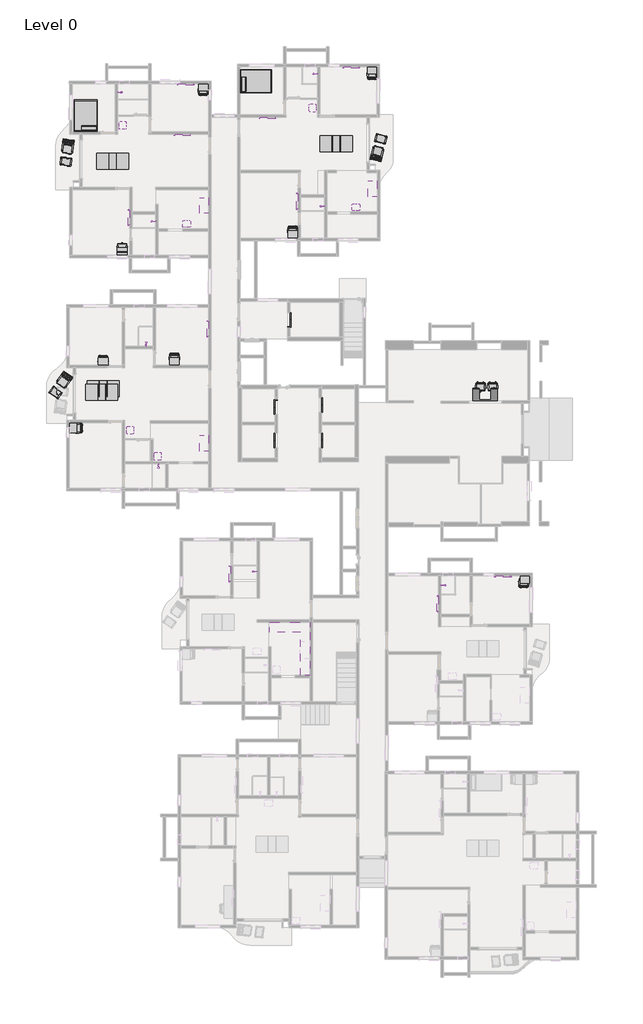
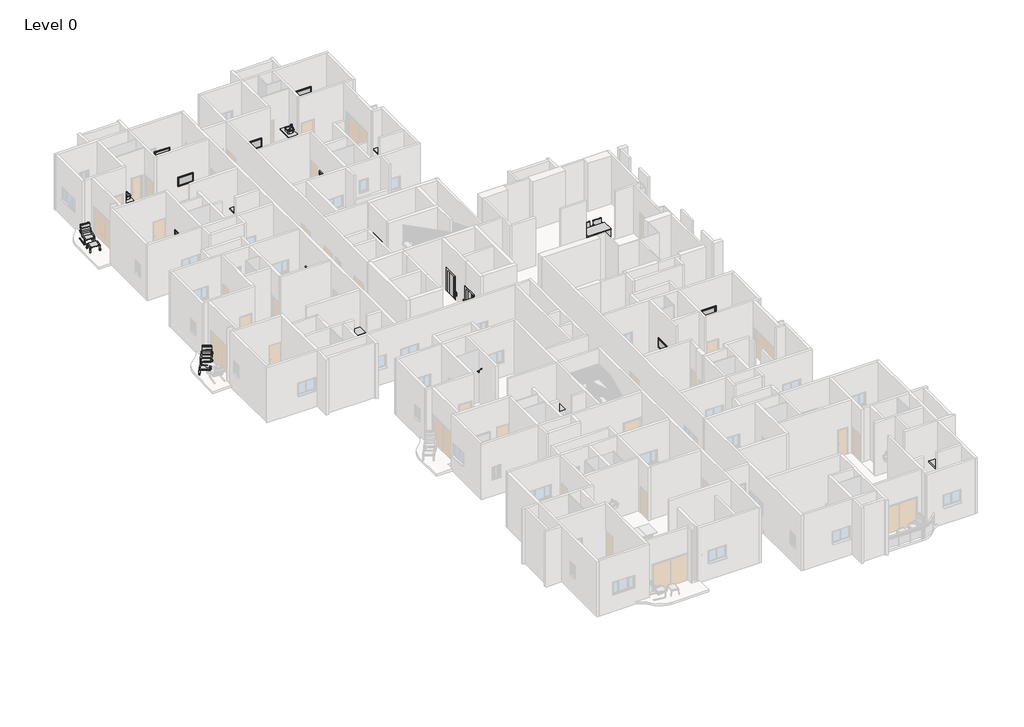
# One storey, part 14 of 14: 40 furniture elements, 14 flow terminals, 9 proxies.
"""IFC4 building model written with IfcOpenShell, lengths in millimetres."""

from ifc_helpers import new_model, si_unit, origin, place, context, project, spatial, transform, mapped, element, save
from components import cook_top_2_0915_x_500mm_892363c5, generic_models_1_generic_models_1_6d9a1767, lift_assembly_13_person_wide_car_39bd1a5e, lift_assembly_13_person_wide_car_ee12aecb, flow_terminal_f629513f, plumbing_fixtures_shower_head_metal_shower_head_9404fff0, furniture_b0964881, escritorio_de_estudiante_de_600x740mm_600_x_460_x_740mm_3f482482, furniture_bed_2_1422x1981x330mm_double_d56b303b, furniture_chair_desk_w_armrest_2_635x686x380mm_bb362225, furniture_desk_1525x762mm_aed207d5, furniture_0b97a49d, furniture_table_dining_w_chairs_rectangular_2000x1000x750mm_b8cbee69

model = new_model("IFC4")

# Units and contexts
model_context = context("Model", 3, world=origin())
ifc_project = project(units=[si_unit("LENGTHUNIT", "METRE", prefix="MILLI")], contexts=[model_context])

# Site, building, storey
site = spatial("IfcSite", under=ifc_project)
building = spatial("IfcBuilding", under=site)
storey = spatial("IfcBuildingStorey", under=building, Name="Level 0", Elevation=0.0)

# Proxies
placement = place(None, origin())
cook_top_2_0915_x_500mm_shape = cook_top_2_0915_x_500mm_892363c5(model_context)
element("IfcBuildingElementProxy", 1, Name="Cook_Top_(2) : 0915 x 500mm", ObjectType="Cook_Top_(2) : 0915 x 500mm", at=placement, inside=storey, context=model_context, shape_type="MappedRepresentation", body=[
    mapped(cook_top_2_0915_x_500mm_shape, transform((-20750.6772109, 57910.8698597, 457.2), x_axis=(0.0, 1.0, 0.0), y_axis=(-1.0, 0.0, 0.0), z_axis=(0.0, 0.0, 1.0))),
])
element("IfcBuildingElementProxy", 2, Name="Cook_Top_(2) : 0915 x 500mm", ObjectType="Cook_Top_(2) : 0915 x 500mm", at=placement, inside=storey, context=model_context, shape_type="MappedRepresentation", body=[
    mapped(cook_top_2_0915_x_500mm_shape, transform((-31256.0679937, 56865.2998557, 457.2), x_axis=(0.0, 1.0, 0.0), y_axis=(-1.0, 0.0, 0.0), z_axis=(0.0, 0.0, 1.0))),
])
element("IfcBuildingElementProxy", 3, Name="Cook_Top_(2) : 0915 x 500mm", ObjectType="Cook_Top_(2) : 0915 x 500mm", at=placement, inside=storey, context=model_context, shape_type="MappedRepresentation", body=[
    mapped(cook_top_2_0915_x_500mm_shape, transform((-31251.7442282, 42057.0998557, 457.2), x_axis=(0.0, 1.0, 0.0), y_axis=(-1.0, 0.0, 0.0), z_axis=(0.0, 0.0, 1.0))),
])
generic_models_1_generic_models_1_shape = generic_models_1_generic_models_1_6d9a1767(model_context)
element("IfcBuildingElementProxy", 4, Name="Generic Models 1 : Generic Models 1", ObjectType="Generic Models 1 : Generic Models 1", at=placement, inside=storey, context=model_context, shape_type="MappedRepresentation", body=[
    mapped(generic_models_1_generic_models_1_shape, transform((0.0, 0.0, 0.0), x_axis=(1.0, 0.0, 0.0), y_axis=(0.0, 1.0, 0.0), z_axis=(0.0, 0.0, 1.0))),
])
lift_assembly_13_person_wide_car_shape = lift_assembly_13_person_wide_car_39bd1a5e(model_context)
element("IfcBuildingElementProxy", 5, Name="Lift_Assembly : 13 Person Wide Car", ObjectType="Lift_Assembly : 13 Person Wide Car", at=placement, inside=storey, context=model_context, shape_type="MappedRepresentation", body=[
    mapped(lift_assembly_13_person_wide_car_shape, transform((-24002.1411875, 41977.5183335, 0.0), x_axis=(0.0, -1.0, 0.0), y_axis=(1.0, 0.0, 0.0), z_axis=(0.0, 0.0, 1.0))),
])
element("IfcBuildingElementProxy", 6, Name="Lift_Assembly : 13 Person Wide Car", ObjectType="Lift_Assembly : 13 Person Wide Car", at=placement, inside=storey, context=model_context, shape_type="MappedRepresentation", body=[
    mapped(lift_assembly_13_person_wide_car_shape, transform((-26762.2514993, 44547.2690597, 0.0), x_axis=(0.0, 1.0, 0.0), y_axis=(-1.0, 0.0, 0.0), z_axis=(0.0, 0.0, 1.0))),
])
element("IfcBuildingElementProxy", 7, Name="Lift_Assembly : 13 Person Wide Car", ObjectType="Lift_Assembly : 13 Person Wide Car", at=placement, inside=storey, context=model_context, shape_type="MappedRepresentation", body=[
    mapped(lift_assembly_13_person_wide_car_shape, transform((-26759.8805211, 42477.5183335, 0.0), x_axis=(0.0, 1.0, 0.0), y_axis=(-1.0, 0.0, 0.0), z_axis=(0.0, 0.0, 1.0))),
])
element("IfcBuildingElementProxy", 8, Name="Lift_Assembly : 13 Person Wide Car", ObjectType="Lift_Assembly : 13 Person Wide Car", at=placement, inside=storey, context=model_context, shape_type="MappedRepresentation", body=[
    mapped(lift_assembly_13_person_wide_car_shape, transform((-25963.5911684, 49491.4513598, 0.0), x_axis=(0.0, -1.0, 0.0), y_axis=(1.0, 0.0, 0.0), z_axis=(0.0, 0.0, 1.0))),
])
lift_assembly_13_person_wide_car_2_shape = lift_assembly_13_person_wide_car_ee12aecb(model_context)
element("IfcBuildingElementProxy", 9, Name="Lift_Assembly : 13 Person Wide Car", ObjectType="Lift_Assembly : 13 Person Wide Car", at=placement, inside=storey, context=model_context, shape_type="MappedRepresentation", body=[
    mapped(lift_assembly_13_person_wide_car_2_shape, transform((-24003.9805211, 44686.2936966, 0.0), x_axis=(0.0, 1.0, 0.0), y_axis=(-1.0, 0.0, 0.0), z_axis=(0.0, 0.0, 1.0))),
])

# Flow terminals
flow_terminal_shape = flow_terminal_f629513f(model_context)
element("IfcFlowTerminal", 10, at=placement, inside=storey, context=model_context, shape_type="MappedRepresentation", body=[
    mapped(flow_terminal_shape, transform((-21776.3879704, 56720.9454557, 762.0), x_axis=(-1.0, 0.0, 0.0), y_axis=(0.0, -1.0, 0.0), z_axis=(0.0, 0.0, 1.0))),
])
element("IfcFlowTerminal", 11, at=placement, inside=storey, context=model_context, shape_type="MappedRepresentation", body=[
    mapped(flow_terminal_shape, transform((-24451.9348422, 62955.7591003, 762.0), x_axis=(0.0, -1.0, 0.0), y_axis=(1.0, 0.0, 0.0), z_axis=(0.0, 0.0, 1.0))),
])
element("IfcFlowTerminal", 12, at=placement, inside=storey, context=model_context, shape_type="MappedRepresentation", body=[
    mapped(flow_terminal_shape, transform((-36372.3794697, 61842.1330151, 762.0), x_axis=(0.0, 1.0, 0.0), y_axis=(-1.0, 0.0, 0.0), z_axis=(0.0, 0.0, 1.0))),
])
element("IfcFlowTerminal", 13, at=placement, inside=storey, context=model_context, shape_type="MappedRepresentation", body=[
    mapped(flow_terminal_shape, transform((-32332.5787531, 55683.937418, 762.0), x_axis=(-1.0, 0.0, 0.0), y_axis=(0.0, -1.0, 0.0), z_axis=(0.0, 0.0, 1.0))),
])
element("IfcFlowTerminal", 14, at=placement, inside=storey, context=model_context, shape_type="MappedRepresentation", body=[
    mapped(flow_terminal_shape, transform((-34180.8635011, 41216.9094066, 762.0), x_axis=(0.0, 1.0, 0.0), y_axis=(-1.0, 0.0, 0.0), z_axis=(0.0, 0.0, 1.0))),
])
element("IfcFlowTerminal", 15, at=placement, inside=storey, context=model_context, shape_type="MappedRepresentation", body=[
    mapped(flow_terminal_shape, transform((-35895.2619011, 42854.2106151, 762.0), x_axis=(0.0, 1.0, 0.0), y_axis=(-1.0, 0.0, 0.0), z_axis=(0.0, 0.0, 1.0))),
])
plumbing_fixtures_shower_head_metal_shower_head_shape = plumbing_fixtures_shower_head_metal_shower_head_9404fff0(model_context)
element("IfcFlowTerminal", 16, ObjectType="Plumbing_Fixtures_Shower_Head : Metal_Shower_Head", at=placement, inside=storey, context=model_context, shape_type="MappedRepresentation", body=[
    mapped(plumbing_fixtures_shower_head_metal_shower_head_shape, transform((-34110.1839022, 40756.2978471, 1369.1616), x_axis=(-1.0, 0.0, 0.0), y_axis=(0.0, -1.0, 0.0), z_axis=(0.0, 0.0, 1.0))),
])
element("IfcFlowTerminal", 17, ObjectType="Plumbing_Fixtures_Shower_Head : Metal_Shower_Head", at=placement, inside=storey, context=model_context, shape_type="MappedRepresentation", body=[
    mapped(plumbing_fixtures_shower_head_metal_shower_head_shape, transform((-34876.5432055, 48089.4982557, 1219.2), x_axis=(1.0, 0.0, 0.0), y_axis=(0.0, 1.0, 0.0), z_axis=(0.0, 0.0, 1.0))),
])
element("IfcFlowTerminal", 18, ObjectType="Plumbing_Fixtures_Shower_Head : Metal_Shower_Head", at=placement, inside=storey, context=model_context, shape_type="MappedRepresentation", body=[
    mapped(plumbing_fixtures_shower_head_metal_shower_head_shape, transform((-27953.0447747, 34054.5800488, 1219.2), x_axis=(0.0, 1.0, 0.0), y_axis=(-1.0, 0.0, 0.0), z_axis=(0.0, 0.0, 1.0))),
])
element("IfcFlowTerminal", 19, ObjectType="Plumbing_Fixtures_Shower_Head : Metal_Shower_Head", at=placement, inside=storey, context=model_context, shape_type="MappedRepresentation", body=[
    mapped(plumbing_fixtures_shower_head_metal_shower_head_shape, transform((-16476.4486976, 33196.3114683, 1369.1616), x_axis=(0.0, -1.0, 0.0), y_axis=(1.0, 0.0, 0.0), z_axis=(0.0, 0.0, 1.0))),
])
element("IfcFlowTerminal", 20, ObjectType="Plumbing_Fixtures_Shower_Head : Metal_Shower_Head", at=placement, inside=storey, context=model_context, shape_type="MappedRepresentation", body=[
    mapped(plumbing_fixtures_shower_head_metal_shower_head_shape, transform((-24192.4144411, 65068.5242932, 1219.2), x_axis=(0.0, 1.0, 0.0), y_axis=(-1.0, 0.0, 0.0), z_axis=(0.0, 0.0, 1.0))),
])
element("IfcFlowTerminal", 21, ObjectType="Plumbing_Fixtures_Shower_Head : Metal_Shower_Head", at=placement, inside=storey, context=model_context, shape_type="MappedRepresentation", body=[
    mapped(plumbing_fixtures_shower_head_metal_shower_head_shape, transform((-23747.8772109, 56814.4794361, 1369.1616), x_axis=(0.0, 1.0, 0.0), y_axis=(-1.0, 0.0, 0.0), z_axis=(0.0, 0.0, 1.0))),
])
element("IfcFlowTerminal", 22, ObjectType="Plumbing_Fixtures_Shower_Head : Metal_Shower_Head", at=placement, inside=storey, context=model_context, shape_type="MappedRepresentation", body=[
    mapped(plumbing_fixtures_shower_head_metal_shower_head_shape, transform((-34278.6679937, 55874.6998557, 1369.1616), x_axis=(0.0, 1.0, 0.0), y_axis=(-1.0, 0.0, 0.0), z_axis=(0.0, 0.0, 1.0))),
])
element("IfcFlowTerminal", 23, ObjectType="Plumbing_Fixtures_Shower_Head : Metal_Shower_Head", at=placement, inside=storey, context=model_context, shape_type="MappedRepresentation", body=[
    mapped(plumbing_fixtures_shower_head_metal_shower_head_shape, transform((-36657.2998709, 63913.7998557, 1369.1616), x_axis=(0.0, -1.0, 0.0), y_axis=(1.0, 0.0, 0.0), z_axis=(0.0, 0.0, 1.0))),
])

# Furniture
furniture_shape = furniture_b0964881(model_context)
element("IfcFurniture", 24, at=placement, inside=storey, context=model_context, shape_type="MappedRepresentation", body=[
    mapped(furniture_shape, transform((-20465.0288109, 60084.2077386, 149.9616), x_axis=(0.9702957262759933, -0.24192189559968053, 0.0), y_axis=(0.24192189559968053, 0.9702957262759933, 0.0), z_axis=(0.0, 0.0, 1.0))),
])
element("IfcFurniture", 25, at=placement, inside=storey, context=model_context, shape_type="MappedRepresentation", body=[
    mapped(furniture_shape, transform((-39747.8075009, 60551.8544135, 149.9616), x_axis=(-0.991992526425774, 0.1262965855255408, 0.0), y_axis=(-0.1262965855255408, -0.991992526425774, 0.0), z_axis=(0.0, 0.0, 1.0))),
])
element("IfcFurniture", 26, at=placement, inside=storey, context=model_context, shape_type="MappedRepresentation", body=[
    mapped(furniture_shape, transform((-39959.6367319, 46005.2866139, 149.9616), x_axis=(-0.8191520442889848, 0.5735764363510562, 0.0), y_axis=(-0.5735764363510562, -0.8191520442889848, 0.0), z_axis=(0.0, 0.0, 1.0))),
])
escritorio_de_estudiante_de_600x740mm_600_x_460_x_740mm_shape = escritorio_de_estudiante_de_600x740mm_600_x_460_x_740mm_3f482482(model_context)
element("IfcFurniture", 27, ObjectType="Escritorio_de_estudiante_de_600x740mm : 600 x 460 x 740mm", at=placement, inside=storey, context=model_context, shape_type="MappedRepresentation", body=[
    mapped(escritorio_de_estudiante_de_600x740mm_600_x_460_x_740mm_shape, transform((-37550.9442282, 47149.6982557, 149.9616), x_axis=(1.0, 0.0, 0.0), y_axis=(0.0, 1.0, 0.0), z_axis=(0.0, 0.0, 1.0))),
])
element("IfcFurniture", 28, ObjectType="Escritorio_de_estudiante_de_600x740mm : 600 x 460 x 740mm", at=placement, inside=storey, context=model_context, shape_type="MappedRepresentation", body=[
    mapped(escritorio_de_estudiante_de_600x740mm_600_x_460_x_740mm_shape, transform((-33105.9442282, 47149.6982557, 149.9616), x_axis=(1.0, 0.0, 0.0), y_axis=(0.0, 1.0, 0.0), z_axis=(0.0, 0.0, 1.0))),
])
element("IfcFurniture", 29, ObjectType="Escritorio_de_estudiante_de_600x740mm : 600 x 460 x 740mm", at=placement, inside=storey, context=model_context, shape_type="MappedRepresentation", body=[
    mapped(escritorio_de_estudiante_de_600x740mm_600_x_460_x_740mm_shape, transform((-39417.0800447, 42996.8998557, 149.9616), x_axis=(0.0, 1.0, 0.0), y_axis=(-1.0, 0.0, 0.0), z_axis=(0.0, 0.0, 1.0))),
])
element("IfcFurniture", 30, ObjectType="Escritorio_de_estudiante_de_600x740mm : 600 x 460 x 740mm", at=placement, inside=storey, context=model_context, shape_type="MappedRepresentation", body=[
    mapped(escritorio_de_estudiante_de_600x740mm_600_x_460_x_740mm_shape, transform((-11240.0417798, 33558.3122683, 149.9616), x_axis=(1.0, 0.0, 0.0), y_axis=(0.0, 1.0, 0.0), z_axis=(0.0, 0.0, 1.0))),
])
element("IfcFurniture", 31, ObjectType="Escritorio_de_estudiante_de_600x740mm : 600 x 460 x 740mm", at=placement, inside=storey, context=model_context, shape_type="MappedRepresentation", body=[
    mapped(escritorio_de_estudiante_de_600x740mm_600_x_460_x_740mm_shape, transform((-25729.0772109, 55064.4250546, 149.9616), x_axis=(1.0, 0.0, 0.0), y_axis=(0.0, 1.0, 0.0), z_axis=(0.0, 0.0, 1.0))),
])
element("IfcFurniture", 32, ObjectType="Escritorio_de_estudiante_de_600x740mm : 600 x 460 x 740mm", at=placement, inside=storey, context=model_context, shape_type="MappedRepresentation", body=[
    mapped(escritorio_de_estudiante_de_600x740mm_600_x_460_x_740mm_shape, transform((-20769.8288109, 65289.6714597, 149.9616), x_axis=(1.0, 0.0, 0.0), y_axis=(0.0, 1.0, 0.0), z_axis=(0.0, 0.0, 1.0))),
])
element("IfcFurniture", 33, ObjectType="Escritorio_de_estudiante_de_600x740mm : 600 x 460 x 740mm", at=placement, inside=storey, context=model_context, shape_type="MappedRepresentation", body=[
    mapped(escritorio_de_estudiante_de_600x740mm_600_x_460_x_740mm_shape, transform((-31302.5442282, 64231.2998557, 149.9616), x_axis=(1.0, 0.0, 0.0), y_axis=(0.0, 1.0, 0.0), z_axis=(0.0, 0.0, 1.0))),
])
element("IfcFurniture", 34, ObjectType="Escritorio_de_estudiante_de_600x740mm : 600 x 460 x 740mm", at=placement, inside=storey, context=model_context, shape_type="MappedRepresentation", body=[
    mapped(escritorio_de_estudiante_de_600x740mm_600_x_460_x_740mm_shape, transform((-36361.4679937, 54002.0170169, 149.9616), x_axis=(1.0, 0.0, 0.0), y_axis=(0.0, 1.0, 0.0), z_axis=(0.0, 0.0, 1.0))),
])
furniture_bed_2_1422x1981x330mm_double_shape = furniture_bed_2_1422x1981x330mm_double_d56b303b(model_context)
element("IfcFurniture", 35, ObjectType="Furniture_Bed_2 : 1422x1981x330mm-Double", at=placement, inside=storey, context=model_context, shape_type="MappedRepresentation", body=[
    mapped(furniture_bed_2_1422x1981x330mm_double_shape, transform((-38649.5958282, 61462.6998557, 149.9616), x_axis=(-1.0, 0.0, 0.0), y_axis=(0.0, -1.0, 0.0), z_axis=(0.0, 0.0, 1.0))),
])
element("IfcFurniture", 36, ObjectType="Furniture_Bed_2 : 1422x1981x330mm-Double", at=placement, inside=storey, context=model_context, shape_type="MappedRepresentation", body=[
    mapped(furniture_bed_2_1422x1981x330mm_double_shape, transform((-29018.4788109, 64631.3498557, 149.9616), x_axis=(0.0, 1.0, 0.0), y_axis=(-1.0, 0.0, 0.0), z_axis=(0.0, 0.0, 1.0))),
])
furniture_chair_desk_w_armrest_2_635x686x380mm_shape = furniture_chair_desk_w_armrest_2_635x686x380mm_bb362225(model_context)
element("IfcFurniture", 37, ObjectType="Furniture_Chair_Desk_w-Armrest_2 : 635x686x380mm", at=placement, inside=storey, context=model_context, shape_type="MappedRepresentation", body=[
    mapped(furniture_chair_desk_w_armrest_2_635x686x380mm_shape, transform((-39093.3341431, 42855.909036, 149.9616), x_axis=(0.0, 1.0, 0.0), y_axis=(-1.0, 0.0, 0.0), z_axis=(0.0, 0.0, 1.0))),
])
element("IfcFurniture", 38, ObjectType="Furniture_Chair_Desk_w-Armrest_2 : 635x686x380mm", at=placement, inside=storey, context=model_context, shape_type="MappedRepresentation", body=[
    mapped(furniture_chair_desk_w_armrest_2_635x686x380mm_shape, transform((-37409.9534085, 47263.9957573, 149.9616), x_axis=(-1.0, 0.0, 0.0), y_axis=(0.0, -1.0, 0.0), z_axis=(0.0, 0.0, 1.0))),
])
element("IfcFurniture", 39, ObjectType="Furniture_Chair_Desk_w-Armrest_2 : 635x686x380mm", at=placement, inside=storey, context=model_context, shape_type="MappedRepresentation", body=[
    mapped(furniture_chair_desk_w_armrest_2_635x686x380mm_shape, transform((-32964.9534085, 47395.2165614, 149.9616), x_axis=(-1.0, 0.0, 0.0), y_axis=(0.0, -1.0, 0.0), z_axis=(0.0, 0.0, 1.0))),
])
element("IfcFurniture", 40, ObjectType="Furniture_Chair_Desk_w-Armrest_2 : 635x686x380mm", at=placement, inside=storey, context=model_context, shape_type="MappedRepresentation", body=[
    mapped(furniture_chair_desk_w_armrest_2_635x686x380mm_shape, transform((-11457.2325995, 33309.3663667, 149.9616), x_axis=(1.0, 0.0, 0.0), y_axis=(0.0, 1.0, 0.0), z_axis=(0.0, 0.0, 1.0))),
])
element("IfcFurniture", 41, ObjectType="Furniture_Chair_Desk_w-Armrest_2 : 635x686x380mm", at=placement, inside=storey, context=model_context, shape_type="MappedRepresentation", body=[
    mapped(furniture_chair_desk_w_armrest_2_635x686x380mm_shape, transform((-13874.8964208, 45604.4149614, 508.1016), x_axis=(-1.0, 0.0, 0.0), y_axis=(0.0, -1.0, 0.0), z_axis=(0.0, 0.0, 1.0))),
])
element("IfcFurniture", 42, ObjectType="Furniture_Chair_Desk_w-Armrest_2 : 635x686x380mm", at=placement, inside=storey, context=model_context, shape_type="MappedRepresentation", body=[
    mapped(furniture_chair_desk_w_armrest_2_635x686x380mm_shape, transform((-13112.8964208, 45604.4149614, 508.1016), x_axis=(-1.0, 0.0, 0.0), y_axis=(0.0, -1.0, 0.0), z_axis=(0.0, 0.0, 1.0))),
])
element("IfcFurniture", 43, ObjectType="Furniture_Chair_Desk_w-Armrest_2 : 635x686x380mm", at=placement, inside=storey, context=model_context, shape_type="MappedRepresentation", body=[
    mapped(furniture_chair_desk_w_armrest_2_635x686x380mm_shape, transform((-25588.0863913, 55313.3709563, 149.9616), x_axis=(-1.0, 0.0, 0.0), y_axis=(0.0, -1.0, 0.0), z_axis=(0.0, 0.0, 1.0))),
])
element("IfcFurniture", 44, ObjectType="Furniture_Chair_Desk_w-Armrest_2 : 635x686x380mm", at=placement, inside=storey, context=model_context, shape_type="MappedRepresentation", body=[
    mapped(furniture_chair_desk_w_armrest_2_635x686x380mm_shape, transform((-20910.8196306, 64991.3255581, 149.9616), x_axis=(1.0, 0.0, 0.0), y_axis=(0.0, 1.0, 0.0), z_axis=(0.0, 0.0, 1.0))),
])
element("IfcFurniture", 45, ObjectType="Furniture_Chair_Desk_w-Armrest_2 : 635x686x380mm", at=placement, inside=storey, context=model_context, shape_type="MappedRepresentation", body=[
    mapped(furniture_chair_desk_w_armrest_2_635x686x380mm_shape, transform((-31443.5350478, 63982.353954, 149.9616), x_axis=(1.0, 0.0, 0.0), y_axis=(0.0, 1.0, 0.0), z_axis=(0.0, 0.0, 1.0))),
])
element("IfcFurniture", 46, ObjectType="Furniture_Chair_Desk_w-Armrest_2 : 635x686x380mm", at=placement, inside=storey, context=model_context, shape_type="MappedRepresentation", body=[
    mapped(furniture_chair_desk_w_armrest_2_635x686x380mm_shape, transform((-36502.4588134, 54186.2711153, 149.9616), x_axis=(1.0, 0.0, 0.0), y_axis=(0.0, 1.0, 0.0), z_axis=(0.0, 0.0, 1.0))),
])
furniture_desk_1525x762mm_shape = furniture_desk_1525x762mm_aed207d5(model_context)
element("IfcFurniture", 47, ObjectType="Furniture_Desk : 1525x762mm", at=placement, inside=storey, context=model_context, shape_type="MappedRepresentation", body=[
    mapped(furniture_desk_1525x762mm_shape, transform((-14498.3110598, 44696.4690597, 508.1016), x_axis=(1.0, 0.0, 0.0), y_axis=(0.0, 1.0, 0.0), z_axis=(0.0, 0.0, 1.0))),
])
furniture_2_shape = furniture_0b97a49d(model_context)
element("IfcFurniture", 48, ObjectType="Furniture_TV_Plasma : 42\"", at=placement, inside=storey, context=model_context, shape_type="MappedRepresentation", body=[
    mapped(furniture_2_shape, transform((-29610.8489269, 33969.5541094, 1369.1616), x_axis=(0.0, -1.0, 0.0), y_axis=(1.0, 0.0, 0.0), z_axis=(0.0, 0.0, 1.0))),
])
element("IfcFurniture", 49, ObjectType="Furniture_TV_Plasma : 42\"", at=placement, inside=storey, context=model_context, shape_type="MappedRepresentation", body=[
    mapped(furniture_2_shape, transform((-12692.6486976, 33786.9122683, 1369.1616), x_axis=(1.0, 0.0, 0.0), y_axis=(0.0, 1.0, 0.0), z_axis=(0.0, 0.0, 1.0))),
])
element("IfcFurniture", 50, ObjectType="Furniture_TV_Plasma : 42\"", at=placement, inside=storey, context=model_context, shape_type="MappedRepresentation", body=[
    mapped(furniture_2_shape, transform((-16628.8486976, 32085.0106683, 1369.1616), x_axis=(0.0, -1.0, 0.0), y_axis=(1.0, 0.0, 0.0), z_axis=(0.0, 0.0, 1.0))),
])
element("IfcFurniture", 51, ObjectType="Furniture_TV_Plasma : 42\"", at=placement, inside=storey, context=model_context, shape_type="MappedRepresentation", body=[
    mapped(furniture_2_shape, transform((-25398.8772109, 57186.9698597, 1369.1616), x_axis=(0.0, -1.0, 0.0), y_axis=(1.0, 0.0, 0.0), z_axis=(0.0, 0.0, 1.0))),
])
element("IfcFurniture", 52, ObjectType="Furniture_TV_Plasma : 42\"", at=placement, inside=storey, context=model_context, shape_type="MappedRepresentation", body=[
    mapped(furniture_2_shape, transform((-27354.7144411, 62364.2982557, 1369.1616), x_axis=(1.0, 0.0, 0.0), y_axis=(0.0, 1.0, 0.0), z_axis=(0.0, 0.0, 1.0))),
])
element("IfcFurniture", 53, ObjectType="Furniture_TV_Plasma : 42\"", at=placement, inside=storey, context=model_context, shape_type="MappedRepresentation", body=[
    mapped(furniture_2_shape, transform((-22135.0788109, 65518.2714597, 1369.1616), x_axis=(1.0, 0.0, 0.0), y_axis=(0.0, 1.0, 0.0), z_axis=(0.0, 0.0, 1.0))),
])
element("IfcFurniture", 54, ObjectType="Furniture_TV_Plasma : 42\"", at=placement, inside=storey, context=model_context, shape_type="MappedRepresentation", body=[
    mapped(furniture_2_shape, transform((-32661.4442282, 61297.4982557, 1369.1616), x_axis=(1.0, 0.0, 0.0), y_axis=(0.0, 1.0, 0.0), z_axis=(0.0, 0.0, 1.0))),
])
element("IfcFurniture", 55, ObjectType="Furniture_TV_Plasma : 42\"", at=placement, inside=storey, context=model_context, shape_type="MappedRepresentation", body=[
    mapped(furniture_2_shape, transform((-35904.2679937, 56173.7170169, 1369.1616), x_axis=(0.0, -1.0, 0.0), y_axis=(1.0, 0.0, 0.0), z_axis=(0.0, 0.0, 1.0))),
])
element("IfcFurniture", 56, ObjectType="Furniture_TV_Plasma : 42\"", at=placement, inside=storey, context=model_context, shape_type="MappedRepresentation", body=[
    mapped(furniture_2_shape, transform((-32458.2442282, 64459.8998557, 1219.2), x_axis=(1.0, 0.0, 0.0), y_axis=(0.0, 1.0, 0.0), z_axis=(0.0, 0.0, 1.0))),
])
element("IfcFurniture", 57, ObjectType="Furniture_TV_Plasma : 42\"", at=placement, inside=storey, context=model_context, shape_type="MappedRepresentation", body=[
    mapped(furniture_2_shape, transform((-30972.3442282, 49232.5998557, 1219.2), x_axis=(0.0, -1.0, 0.0), y_axis=(1.0, 0.0, 0.0), z_axis=(0.0, 0.0, 1.0))),
])
element("IfcFurniture", 58, ObjectType="Furniture_TV_Plasma : 42\"", at=placement, inside=storey, context=model_context, shape_type="MappedRepresentation", body=[
    mapped(furniture_2_shape, transform((-16628.8486976, 32110.4106683, 1369.1616), x_axis=(0.0, -1.0, 0.0), y_axis=(1.0, 0.0, 0.0), z_axis=(0.0, 0.0, 1.0))),
])
element("IfcFurniture", 59, ObjectType="Furniture_TV_Plasma : 42\"", at=placement, inside=storey, context=model_context, shape_type="MappedRepresentation", body=[
    mapped(furniture_2_shape, transform((-12641.8486976, 33786.9122683, 1369.1616), x_axis=(1.0, 0.0, 0.0), y_axis=(0.0, 1.0, 0.0), z_axis=(0.0, 0.0, 1.0))),
])
furniture_table_dining_w_chairs_rectangular_2000x1000x750mm_shape = furniture_table_dining_w_chairs_rectangular_2000x1000x750mm_b8cbee69(model_context)
element("IfcFurniture", 60, ObjectType="Furniture_Table_Dining_w-Chairs_Rectangular : 2000x1000x750mm_w-6_Seats", at=placement, inside=storey, context=model_context, shape_type="MappedRepresentation", body=[
    mapped(furniture_table_dining_w_chairs_rectangular_2000x1000x750mm_shape, transform((-37757.2587666, 45194.0952265, 149.9616), x_axis=(1.0, 0.0, 0.0), y_axis=(0.0, 1.0, 0.0), z_axis=(0.0, 0.0, 1.0))),
])
element("IfcFurniture", 61, ObjectType="Furniture_Table_Dining_w-Chairs_Rectangular : 2000x1000x750mm_w-6_Seats", at=placement, inside=storey, context=model_context, shape_type="MappedRepresentation", body=[
    mapped(furniture_table_dining_w_chairs_rectangular_2000x1000x750mm_shape, transform((-23129.4559328, 60656.3452265, 149.9616), x_axis=(1.0, 0.0, 0.0), y_axis=(0.0, 1.0, 0.0), z_axis=(0.0, 0.0, 1.0))),
])
element("IfcFurniture", 62, ObjectType="Furniture_Table_Dining_w-Chairs_Rectangular : 2000x1000x750mm_w-6_Seats", at=placement, inside=storey, context=model_context, shape_type="MappedRepresentation", body=[
    mapped(furniture_table_dining_w_chairs_rectangular_2000x1000x750mm_shape, transform((-37072.32455, 59589.5452265, 149.9616), x_axis=(1.0, 0.0, 0.0), y_axis=(0.0, 1.0, 0.0), z_axis=(0.0, 0.0, 1.0))),
])
element("IfcFurniture", 63, ObjectType="Furniture_Table_Dining_w-Chairs_Rectangular : 2000x1000x750mm_w-6_Seats", at=placement, inside=storey, context=model_context, shape_type="MappedRepresentation", body=[
    mapped(furniture_table_dining_w_chairs_rectangular_2000x1000x750mm_shape, transform((-37669.12295, 45388.7144305, 149.9616), x_axis=(1.0, 0.0, 0.0), y_axis=(0.0, 1.0, 0.0), z_axis=(0.0, 0.0, 1.0))),
])

save(model, "model.ifc")

# Revit data of these elements
# Type "Cook_Top_(2) : 0915 x 500mm"
#   Keynote = "N"
#   Depth = 500 mm
#   Width = 915 mm
#   Material Burner = Metal - Chrome
#   Material Cooktop = Metal - Steel, Polished
#   Default Elevation = 0
# Type "Lift_Assembly : 13 Person Wide Car"
#   Keynote = "X"
#   Hoistway Width = 2400 mm
#   Hoistway Depth = 1800 mm
#   Height = 2100 mm
#   Frame Width = 75 mm
#   Percentage Opened (Plan) = 0 mm
#   Door Width = 900 mm
#   Door Trim Width = 100 mm
#   Door Thickness = 50 mm
#   Car Width = 1600 mm
#   Car Thickness = 25 mm
#   Car Front Offset = 250 mm
#   Car Depth = 1400 mm
#   Call Point Z Offset = 1000 mm
#   Call Point X Offset = 200 mm
#   Call Point Panel Width = 150 mm
#   Call Point Panel Depth = 250 mm
#   Vis - Hoistway Location Lines = yes
#   Vis - Door Trim = yes
#   Vis - Call Point = yes
#   Material Trim = Metal - Stainless Steel
#   Material Doors = Metal - Aluminium
#   Wall Closure = (empty or 0)
#   Default Elevation = 0
# Type
#   Hauteur du plan de travail = 750 mm
#   Profondeur = 440 mm
#   Largeur = 500 mm
#   Default Elevation = 0
# Type "Plumbing_Fixtures_Shower_Head : Metal_Shower_Head"
#   Keynote = "N13/230"
#   Mounting Height = 1600 mm
#   Material Shower Head = Metal - Chrome Polished
#   Default Elevation = 0
# Type
#   Default Elevation = 0
# Type "Escritorio_de_estudiante_de_600x740mm : 600 x 460 x 740mm"
#   ID_Source = "BIMTOOL"
#   ID_Objeto = "BT_F_G_836"
#   BT_Web_del_Producto = "http://www.bimtool.com/Catalog.aspx?categoria=ESCRITORIOS"
#   BT_Uso = "Interior"
#   BT_SKU = "00 00 00"
#   BT_Profundidad = "460mm"
#   BT_Peso = "N/a"
#   BT_Nombre_Técnico = "Escritorio de estudiante de 600x740mm"
#   BT_Nombre_Corto = "Escritorio de estudiante de 600x740mm"
#   BT_Material = "Madera - Acero"
#   BT_MasterFormat® = "12 00 00"
#   BT_Marca = "Bimtool"
#   BT_Itemizado_Estandar_CDT = "H 06 06 00"
#   BT_Fabricante = "Bimtool"
#   BT_Especialidad = "Mobiliario e Interiorismo"
#   BT_Elemento = "Escritorios"
#   BT_EETT = "Escritorio de estudiante de 600x740mm, con 4 apoyos de acero"
#   BT_Descripción = "Escritorio de madera"
#   BT_Código_Origen = ""
#   BT_Código_Línea = "Línea"
#   BT_Color = "N/a"
#   BT_Ancho = "600mm"
#   BT_Alto = "740mm"
#   Depth = 460 mm
#   Height = 740 mm
#   Width = 600 mm
#   Default Elevation = 0
#   Assembly Code = ""
# Type "Furniture_Bed_2 : 1422x1981x330mm-Double"
#   Keynote = "N"
#   Length = 1981.2 mm
#   Width = 1422.4 mm
#   Material Frame = Wood - Birch
#   Material Mattress = Textile - White
#   Default Elevation = 0
# Type "Furniture_Chair_Desk_w-Armrest_2 : 635x686x380mm"
#   Assembly Code = "E2020200"
#   Material Base = Plastic - Black
#   Material Caster = Plastic - Black
#   Material Seat/Back = Textile - Slate Blue
#   Default Elevation = 0
# Type "Furniture_Desk : 1525x762mm"
#   Keynote = "N"
#   Width = 1525 mm
#   Leg Height = 152 mm
#   Height = 762 mm
#   Depth = 762 mm
#   Top Material = Cherry
#   Handle/Leg Material = Steel, Chrome Plated
#   Body Material = Laminate, Ivory, Matte
#   Default Elevation = 0
#   Assembly Code = ""
# Type "Furniture_TV_Plasma : 42\""
#   Keynote = "N"
#   Assembly Code = "E2020200"
#   Depth = 88.9 mm
#   Height = 660.4 mm
#   Width = 1028.7 mm
#   Material Cabinet = Plastic - Gray
#   Default Elevation = 0
# Type "Furniture_Table_Dining_w-Chairs_Rectangular : 2000x1000x750mm_w-6_Seats"
#   Keynote = "N"
#   Width = 1000 mm
#   Table Top Thickness = 40 mm
#   Table Height = 750 mm
#   Length = 2000 mm
#   Leg Width = 75 mm
#   Leg Spacing Width = 800 mm
#   Leg Spacing Length = 1400 mm
#   Chair Side Spacing = 700 mm
#   Centre Piece = 500 mm
#   Vis - End Chairs = yes
#   Material Table = Wood - Birch
#   Material Chair Structure = Wood - Birch
#   Material Chair Covering = Fabric - Beige
#   Default Elevation = 0
# Elements 1, 2, 3 (IfcBuildingElementProxy, "Cook_Top_(2) : 0915 x 500mm")
#   Phase Created = New Construction
#   Materials on its faces: "Metal - Chrome", "Metal - Steel, Polished"
# Element 4 (IfcBuildingElementProxy, "Generic Models 1 : Generic Models 1")
#   Phase Created = New Construction
#   Materials on its faces: "OUTDOOR FLOORING"
# Elements 5, 6, 7, 8, 9 (IfcBuildingElementProxy, "Lift_Assembly : 13 Person Wide Car")
#   Phase Created = New Construction
#   Materials on its faces: "Metal - Stainless Steel", "Metal - Aluminium"
# Elements 10, 11, 12, 13, 14, 15 (IfcFlowTerminal)
#   Phase Created = New Construction
# Elements 16, 17, 18, 19, 20, 21, 22, 23 (IfcFlowTerminal, "Plumbing_Fixtures_Shower_Head : Metal_Shower_Head")
#   Phase Created = New Construction
#   Materials on its faces: "Metal - Chrome Polished"
# Elements 24, 25, 26 (IfcFurniture)
#   Phase Created = New Construction
#   Materials on its faces: "Wood", "cushion"
# Elements 27, 28, 29, 30, 31, 32, 33, 34 (IfcFurniture, "Escritorio_de_estudiante_de_600x740mm : 600 x 460 x 740mm")
#   Phase Created = New Construction
#   Materials on its faces: "Metal - Chrome", "Wood - Birch", "Metal - Steel"
# Elements 35, 36 (IfcFurniture, "Furniture_Bed_2 : 1422x1981x330mm-Double")
#   Phase Created = New Construction
#   Materials on its faces: "Wood - Birch", "Textile - White"
# Elements 37, 38, 39, 40, 41, 42, 43, 44, 45, 46 (IfcFurniture, "Furniture_Chair_Desk_w-Armrest_2 : 635x686x380mm")
#   Phase Created = New Construction
#   Materials on its faces: "Plastic - Black", "Textile - Slate Blue"
# Element 47 (IfcFurniture, "Furniture_Desk : 1525x762mm")
#   Phase Created = New Construction
#   Materials on its faces: "Steel, Chrome Plated", "Laminate, Ivory, Matte", "Cherry"
# Elements 48, 49, 50, 51, 52, 53, 54, 55, 56, 57, 58, 59 (IfcFurniture, "Furniture_TV_Plasma : 42\"")
#   Phase Created = New Construction
#   Materials on its faces: "Plastic - Black", "Plastic - Gray", "Glass"
# Elements 60, 61, 62, 63 (IfcFurniture, "Furniture_Table_Dining_w-Chairs_Rectangular : 2000x1000x750mm_w-6_Seats")
#   Phase Created = New Construction
#   Materials on its faces: "Wood - Birch"
# Materials
#   "Metal - Chrome": colour RGB 201 201 201, transparency 0
#   "Metal - Steel, Polished": colour RGB 247 247 247, transparency 0
#   "Metal - Stainless Steel": class "Metal", colour RGB 247 247 247, transparency 0
#   "Metal - Aluminium": class "Metal", colour RGB 247 247 247, transparency 0
#   "Metal - Chrome Polished": colour RGB 247 247 247, transparency 0
#   "Wood - Birch": colour RGB 210 159 95, transparency 0
#   "Textile - White": class "Fabric", colour RGB 247 247 239, transparency 0
#   "Plastic - Black": colour RGB 0 0 0, transparency 0
#   "Textile - Slate Blue": class "Fabric", colour RGB 98 102 118, transparency 0
#   "Cherry": class "Wood", colour RGB 226 177 128, transparency 0, Description = "Prunus Serotina", Cost = 0
#   "Steel, Chrome Plated": class "Metal", colour RGB 216 216 216, transparency 0, Description = "Chromiuim plated steel", Cost = 0
#   "Laminate, Ivory, Matte": class "Plastic", colour RGB 247 247 239, transparency 0, Description = "Plastic Laminate - Ivory, Matte", Cost = 0
#   "Plastic - Gray": class "Plastic", colour RGB 134 134 134, transparency 0
#   "Fabric - Beige": class "Fabric", colour RGB 231 227 195, transparency 0
#   "OUTDOOR FLOORING": class "Generic", colour RGB 120 120 120, transparency 0, Cost = 0
#   "Wood": class "Wood", colour RGB 212 179 113, transparency 0, Description = "Generic wood", Cost = 0
#   "cushion": class "Fabric", colour RGB 78 81 77, transparency 0
#   "Metal - Steel": colour RGB 247 247 247, transparency 0
#   "Glass": class "Glass", colour RGB 0 128 192, transparency 0.9, Description = "Soda Lime Glass", Cost = 0
